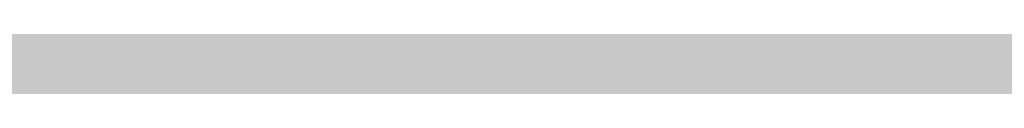
# Model space of a CAD drawing. Units: feet. Extents: x 3168 to 4724, y 827 to 1477.
# Tile 113 of 256: x 3284.48 to 3298.68, y 1098.34 to 1099. Entities that reach past the tile are written whole.
import ezdxf

# ---------------------------------------------------------------- set-up
doc = ezdxf.new("R2010")
doc.units = ezdxf.units.FT
doc.layers.add('A-ELEV', color=7, linetype='Continuous', lineweight=35)
doc.layers.add('A-ELEV-PATT', color=8, linetype='Continuous', lineweight=13)

msp = doc.modelspace()

# ---------------------------------------------------------------- hatches: boundary and pattern name
at = {"layer": 'A-ELEV-PATT'}
h = msp.add_hatch(color=256, dxfattribs=at)
h.dxf.hatch_style = 1
edge = h.paths.add_edge_path()
edge.add_ellipse((3552.906, 979.22), major_axis=(36.745, 0), ratio=0.484848, start_angle=0, end_angle=360)
edge = h.paths.add_edge_path()
edge.add_ellipse((3559.892, 929.252), major_axis=(36.745, 0), ratio=0.484848, start_angle=0, end_angle=360)
edge = h.paths.add_edge_path()
edge.add_line((3299.317, 1198.606), (3479.917, 1198.606))
edge.add_line((3479.917, 1198.606), (3479.917, 1209.869))
edge.add_spline(control_points=[(3479.917, 1209.869), (3464.301, 1209.869), (3448.686, 1209.869), (3410.949, 1209.869), (3388.828, 1209.869), (3355.647, 1209.869), (3344.586, 1209.869), (3327.996, 1209.869), (3322.466, 1209.869), (3314.17, 1209.869), (3311.405, 1209.869), (3307.257, 1209.869), (3305.875, 1209.869), (3303.801, 1209.869), (3303.11, 1209.869), (3302.073, 1209.869), (3301.727, 1209.869), (3301.209, 1209.869), (3301.036, 1209.869), (3300.777, 1209.869), (3300.69, 1209.869), (3300.561, 1209.869), (3300.517, 1209.869), (3300.453, 1209.869), (3300.431, 1209.869), (3300.399, 1209.869), (3300.388, 1209.869), (3300.366, 1209.869), (3300.346, 1209.869), (3300.346, 1209.869), (3300.346, 1209.869), (3300.343, 1209.869), (3300.341, 1209.869), (3300.338, 1209.869), (3300.337, 1209.869), (3300.334, 1209.869), (3300.332, 1209.869), (3300.326, 1209.869), (3300.321, 1209.869), (3300.311, 1209.869), (3300.306, 1209.869), (3300.291, 1209.869), (3300.28, 1209.869), (3300.232, 1209.869), (3300.195, 1209.869), (3299.951, 1209.871), (3299.745, 1209.874), (3299.437, 1209.883), (3299.334, 1209.887), (3299.181, 1209.893), (3299.13, 1209.895), (3298.652, 1209.917), (3298.229, 1209.946), (3297.602, 1210.002), (3297.393, 1210.023), (3297.083, 1210.058), (3296.979, 1210.07), (3296.293, 1210.155), (3295.718, 1210.243), (3294.869, 1210.399), (3294.588, 1210.454), (3294.169, 1210.543), (3294.03, 1210.574), (3291.707, 1211.101), (3289.654, 1211.813), (3285.776, 1213.564), (3283.951, 1214.603), (3280.512, 1216.98), (3278.897, 1218.318), (3276.38, 1220.829), (3275.416, 1221.918), (3274.039, 1223.708), (3273.581, 1224.35), (3273.143, 1225.016)], knot_values=[39.119033, 39.119033, 39.119033, 39.119033, 39.286353, 39.286353, 39.523379, 39.523379, 39.641892, 39.641892, 39.701148, 39.701148, 39.730777, 39.730777, 39.745591, 39.745591, 39.752998, 39.752998, 39.756701, 39.756701, 39.758553, 39.758553, 39.759479, 39.759479, 39.759942, 39.759942, 39.760173, 39.760173, 39.760289, 39.760289, 39.760405, 39.760405, 39.760463, 39.760463, 39.763389, 39.763389, 39.764851, 39.764851, 39.767304, 39.767304, 39.773825, 39.773825, 39.78057, 39.78057, 39.79477, 39.79477, 39.845194, 39.845194, 40.126715, 40.126715, 40.267476, 40.267476, 40.337856, 40.337856, 40.927023, 40.927023, 41.221606, 41.221606, 41.368898, 41.368898, 42.202622, 42.202622, 42.619485, 42.619485, 42.827916, 42.827916, 46.118323, 46.118323, 49.408731, 49.408731, 52.699139, 52.699139, 54.927489, 54.927489, 56.104228, 56.104228, 56.104228, 56.104228], weights=[1, 1, 1, 1, 1, 1, 1, 1, 1, 1, 1, 1, 1, 1, 1, 1, 1, 1, 1, 1, 1, 1, 1, 1, 1, 1, 1, 1, 1, 1, 1, 1, 1, 1, 1, 1, 1, 1, 1, 1, 1, 1, 1, 1, 1, 1, 1, 1, 1, 1, 1, 1, 1, 1, 1, 1, 1, 1, 1, 1, 1, 1, 1, 1, 1, 1, 1, 1, 1, 1, 1, 1, 1, 1], degree=3, periodic=0)
edge.add_line((3273.143, 1225.016), (3273.143, 1099.016))
edge.add_line((3273.143, 1099.016), (3299.317, 1099.016))
edge.add_line((3299.317, 1099.016), (3299.317, 1198.606))
edge = h.paths.add_edge_path()
edge.add_line((3304.758, 1324.158), (3479.917, 1324.158))
edge.add_line((3479.917, 1324.158), (3479.917, 1335.715))
edge.add_line((3479.917, 1335.715), (3269.162, 1335.715))
edge.add_spline(control_points=[(3269.162, 1335.715), (3264.024, 1335.715), (3258.364, 1328.958), (3259.264, 1323.9)], knot_values=[0, 0, 0, 0, 15.412191, 15.412191, 15.412191, 15.412191], degree=3, periodic=0)
edge.add_line((3259.264, 1323.9), (3265.517, 1288.769))
edge.add_line((3265.517, 1288.769), (3275.265, 1261.546))
edge.add_line((3275.265, 1261.546), (3304.758, 1261.546))
edge.add_line((3304.758, 1261.546), (3304.758, 1324.158))
h = msp.add_hatch(color=256, dxfattribs=at)
h.dxf.hatch_style = 1
h.paths.add_polyline_path([(3384.525, 1099.016), (3335.029, 1099.016), (3299.317, 1099.016), (3273.143, 1099.016), (3217.565, 1099.016), (3168.069, 827.116), (3335.029, 827.116)])

# ---------------------------------------------------------------- linework, layer by layer
at = {"layer": 'A-ELEV'}
msp.add_open_spline([(3808.52, 1099.016), (3808.52, 1141.413), (3808.52, 1183.81), (3808.52, 1226.635), (3808.52, 1227.064), (3808.52, 1227.492), (3811.492, 1248.995), (3814.464, 1270.498), (3817.465, 1292.218), (3817.495, 1292.435), (3817.525, 1292.652), (3817.573, 1310.107), (3817.62, 1327.562), (3817.668, 1345.016), (3817.668, 1345.458), (3817.668, 1345.9), (3817.668, 1346.456), (3817.668, 1346.571), (3817.668, 1346.753), (3817.668, 1346.82), (3817.668, 1346.935), (3817.668, 1346.982), (3817.668, 1347.039), (3817.668, 1347.047), (3817.668, 1347.074), (3817.668, 1347.059), (3817.668, 1347.062), (3817.668, 1347.063), (3817.668, 1347.066), (3817.668, 1347.068), (3817.668, 1347.075), (3817.668, 1347.079), (3817.668, 1347.093), (3817.668, 1347.102), (3817.668, 1347.129), (3817.668, 1347.147), (3817.667, 1347.2), (3817.667, 1347.236), (3817.666, 1347.343), (3817.665, 1347.415), (3817.661, 1347.628), (3817.657, 1347.77), (3817.64, 1348.192), (3817.624, 1348.472), (3817.559, 1349.3), (3817.496, 1349.841), (3817.255, 1351.424), (3817.026, 1352.429), (3816.307, 1354.889), (3815.744, 1356.269), (3814.464, 1358.819), (3813.746, 1359.991), (3812.196, 1362.172), (3811.362, 1363.182), (3809.589, 1365.069), (3808.649, 1365.946), (3806.654, 1367.58), (3805.6, 1368.336), (3803.353, 1369.722), (3802.161, 1370.352), (3799.601, 1371.454), (3798.233, 1371.925), (3795.28, 1372.635), (3793.693, 1372.872), (3791.869, 1372.926), (3791.741, 1372.929), (3791.353, 1372.934), (3791.093, 1372.933), (3790.304, 1372.915), (3789.77, 1372.884), (3789.209, 1372.83), (3789.191, 1372.828), (3789.135, 1372.823), (3789.098, 1372.819), (3789.048, 1372.814), (3789.036, 1372.813), (3789, 1372.809), (3788.976, 1372.806), (3788.949, 1372.803), (3788.947, 1372.803), (3788.943, 1372.803), (3788.941, 1372.802), (3788.939, 1372.802), (3788.938, 1372.802), (3788.935, 1372.802), (3788.868, 1372.794), (3788.757, 1372.782), (3788.702, 1372.776), (3788.536, 1372.758), (3788.425, 1372.746), (3788.093, 1372.709), (3787.872, 1372.685), (3787.208, 1372.612), (3786.765, 1372.563), (3785.437, 1372.417), (3784.551, 1372.32), (3781.895, 1372.027), (3780.125, 1371.833), (3774.813, 1371.248), (3771.271, 1370.859), (3760.647, 1369.69), (3753.564, 1368.911), (3732.316, 1366.573), (3718.15, 1365.015), (3694.007, 1362.359), (3684.029, 1361.262), (3674.051, 1360.164), (3664.601, 1360.164), (3655.151, 1360.164), (3626.801, 1360.164), (3607.901, 1360.164), (3551.202, 1360.164), (3513.402, 1360.164), (3467.725, 1360.164), (3459.848, 1360.164), (3436.215, 1360.164), (3420.46, 1360.164), (3373.194, 1360.164), (3341.684, 1360.164), (3302.848, 1360.164), (3295.523, 1360.164), (3286.038, 1360.164), (3283.879, 1360.164), (3277.403, 1360.164), (3273.085, 1360.164), (3267.733, 1360.164), (3266.699, 1360.164), (3263.597, 1360.164), (3261.528, 1360.164), (3259.237, 1360.164), (3259.014, 1360.164), (3258.344, 1360.164), (3257.897, 1360.164), (3257.431, 1360.164), (3257.411, 1360.164), (3257.371, 1360.164), (3257.375, 1360.164), (3257.375, 1360.164), (3257.374, 1360.164), (3257.372, 1360.164), (3257.371, 1360.164), (3257.367, 1360.164), (3257.364, 1360.164), (3257.356, 1360.164), (3257.351, 1360.164), (3257.335, 1360.164), (3257.324, 1360.164), (3257.293, 1360.164), (3257.272, 1360.164), (3257.208, 1360.163), (3257.166, 1360.163), (3257.04, 1360.161), (3256.956, 1360.16), (3256.706, 1360.153), (3256.539, 1360.147), (3256.044, 1360.122), (3255.717, 1360.097), (3254.752, 1360), (3254.128, 1359.907), (3252.18, 1359.525), (3250.942, 1359.144), (3248.67, 1358.243), (3247.636, 1357.724), (3245.733, 1356.603), (3244.863, 1356.002), (3243.253, 1354.743), (3242.512, 1354.085), (3240.751, 1352.345), (3239.801, 1351.23), (3238.088, 1348.872), (3237.325, 1347.63), (3235.983, 1344.972), (3235.402, 1343.555), (3234.591, 1340.815), (3234.311, 1339.544), (3233.976, 1336.803), (3233.922, 1335.331), (3234.149, 1332.591), (3234.35, 1331.367), (3234.72, 1329.999), (3234.752, 1329.883), (3234.854, 1329.535), (3234.926, 1329.302), (3235.025, 1329.003), (3235.047, 1328.937), (3235.078, 1328.847), (3235.086, 1328.823), (3235.111, 1328.751), (3235.128, 1328.703), (3235.148, 1328.646), (3235.151, 1328.638), (3235.156, 1328.624), (3235.158, 1328.618), (3235.16, 1328.612), (3235.166, 1328.597), (3235.18, 1328.556), (3235.19, 1328.528), (3235.221, 1328.443), (3235.241, 1328.386), (3235.302, 1328.216), (3235.343, 1328.102), (3235.465, 1327.762), (3235.546, 1327.535), (3235.79, 1326.853), (3235.953, 1326.399), (3236.44, 1325.037), (3236.766, 1324.128), (3237.741, 1321.403), (3238.392, 1319.587), (3240.344, 1314.137), (3241.645, 1310.504), (3245.548, 1299.604), (3248.15, 1292.337), (3255.956, 1270.537), (3261.16, 1256.004), (3267.388, 1238.612), (3268.411, 1235.753), (3269.51, 1232.684), (3269.586, 1232.474), (3269.707, 1232.136), (3269.752, 1232.008), (3269.827, 1231.799), (3269.856, 1231.718), (3269.906, 1231.578), (3269.927, 1231.52), (3269.972, 1231.393), (3269.997, 1231.325), (3270.027, 1231.243), (3270.032, 1231.228), (3270.04, 1231.204), (3270.039, 1231.207), (3270.039, 1231.207), (3270.039, 1231.206), (3270.04, 1231.206), (3270.04, 1231.205), (3270.04, 1231.204), (3270.04, 1231.204), (3270.041, 1231.201), (3270.042, 1231.2), (3270.043, 1231.195), (3270.045, 1231.192), (3270.048, 1231.183), (3270.05, 1231.177), (3270.056, 1231.159), (3270.061, 1231.147), (3270.074, 1231.111), (3270.083, 1231.087), (3270.109, 1231.014), (3270.127, 1230.966), (3270.18, 1230.822), (3270.216, 1230.727), (3270.325, 1230.442), (3270.4, 1230.253), (3270.629, 1229.691), (3270.789, 1229.324), (3271.286, 1228.238), (3271.643, 1227.54), (3272.776, 1225.515), (3273.614, 1224.261), (3275.416, 1221.918), (3276.38, 1220.829), (3278.897, 1218.318), (3280.512, 1216.98), (3283.951, 1214.603), (3285.776, 1213.564), (3289.654, 1211.813), (3291.707, 1211.101), (3294.03, 1210.574), (3294.169, 1210.543), (3294.588, 1210.454), (3294.869, 1210.399), (3295.718, 1210.243), (3296.293, 1210.155), (3296.979, 1210.07), (3297.083, 1210.058), (3297.393, 1210.023), (3297.602, 1210.002), (3298.229, 1209.946), (3298.652, 1209.917), (3299.13, 1209.895), (3299.181, 1209.893), (3299.334, 1209.887), (3299.437, 1209.883), (3299.745, 1209.874), (3299.951, 1209.871), (3300.195, 1209.869), (3300.232, 1209.869), (3300.28, 1209.869), (3300.291, 1209.869), (3300.306, 1209.869), (3300.311, 1209.869), (3300.321, 1209.869), (3300.326, 1209.869), (3300.332, 1209.869), (3300.334, 1209.869), (3300.337, 1209.869), (3300.338, 1209.869), (3300.341, 1209.869), (3300.343, 1209.869), (3300.346, 1209.869), (3300.346, 1209.869), (3300.346, 1209.869), (3300.366, 1209.869), (3300.388, 1209.869), (3300.399, 1209.869), (3300.431, 1209.869), (3300.453, 1209.869), (3300.517, 1209.869), (3300.561, 1209.869), (3300.69, 1209.869), (3300.777, 1209.869), (3301.036, 1209.869), (3301.209, 1209.869), (3301.727, 1209.869), (3302.073, 1209.869), (3303.11, 1209.869), (3303.801, 1209.869), (3305.875, 1209.869), (3307.257, 1209.869), (3311.405, 1209.869), (3314.17, 1209.869), (3322.466, 1209.869), (3327.996, 1209.869), (3344.586, 1209.869), (3355.647, 1209.869), (3388.828, 1209.869), (3410.949, 1209.869), (3477.312, 1209.869), (3521.554, 1209.869), (3566.836, 1209.869), (3567.877, 1209.869), (3570.999, 1209.869), (3573.08, 1209.869), (3575.781, 1209.869), (3576.401, 1209.869), (3577.296, 1209.869), (3577.571, 1209.869), (3578.397, 1209.869), (3578.948, 1209.869), (3579.756, 1209.869), (3580.015, 1209.869), (3580.343, 1209.869), (3580.327, 1209.869), (3580.327, 1209.869), (3580.327, 1209.869), (3580.328, 1209.869), (3580.328, 1209.869), (3580.329, 1209.869), (3580.33, 1209.869), (3580.331, 1209.869), (3580.333, 1209.869), (3580.336, 1209.869), (3580.339, 1209.869), (3580.346, 1209.869), (3580.351, 1209.869), (3580.366, 1209.869), (3580.375, 1209.869), (3580.405, 1209.868), (3580.424, 1209.868), (3580.483, 1209.868), (3580.522, 1209.868), (3580.64, 1209.867), (3580.719, 1209.865), (3580.956, 1209.861), (3581.115, 1209.856), (3581.594, 1209.837), (3581.916, 1209.818), (3582.89, 1209.742), (3583.548, 1209.666), (3585.532, 1209.361), (3586.867, 1209.054), (3589.472, 1208.252), (3590.74, 1207.758), (3591.995, 1207.159), (3592.058, 1207.129), (3592.244, 1207.038), (3592.368, 1206.977), (3592.735, 1206.79), (3592.977, 1206.663), (3593.245, 1206.516), (3593.275, 1206.5), (3593.365, 1206.45), (3593.425, 1206.416), (3593.604, 1206.315), (3593.723, 1206.247), (3593.857, 1206.168), (3593.874, 1206.158), (3593.926, 1206.128), (3593.96, 1206.108), (3594.062, 1206.047), (3594.13, 1206.006), (3594.208, 1205.958), (3594.22, 1205.951), (3594.253, 1205.931), (3594.276, 1205.917), (3594.343, 1205.876), (3594.388, 1205.848), (3594.434, 1205.819), (3594.435, 1205.818), (3594.44, 1205.815), (3594.443, 1205.813), (3594.447, 1205.811), (3594.448, 1205.81), (3594.449, 1205.81), (3594.449, 1205.809), (3594.45, 1205.809), (3594.45, 1205.808), (3594.451, 1205.808), (3594.467, 1205.798), (3594.493, 1205.782), (3594.506, 1205.774), (3594.545, 1205.749), (3594.571, 1205.733), (3594.648, 1205.684), (3594.7, 1205.652), (3594.855, 1205.555), (3594.959, 1205.49), (3595.269, 1205.295), (3595.476, 1205.166), (3596.097, 1204.776), (3596.511, 1204.517), (3597.753, 1203.739), (3598.581, 1203.22), (3601.064, 1201.664), (3602.72, 1200.626), (3607.687, 1197.513), (3610.998, 1195.438), (3620.932, 1189.212), (3627.555, 1185.061), (3647.423, 1172.61), (3660.668, 1164.309), (3700.403, 1139.405), (3726.894, 1122.803), (3757.206, 1103.806), (3761.027, 1101.411), (3764.848, 1099.016), (3745.328, 1099.016), (3725.808, 1099.016), (3706.288, 1099.016), (3706.288, 1108.453), (3706.288, 1117.89), (3706.288, 1127.327), (3710.751, 1127.327), (3715.213, 1127.327), (3719.676, 1127.327)], degree=3, knots=[0, 0, 0, 0, 0.982037, 0.982037, 0.991957, 0.991957, 0.991957, 1.966522, 1.966522, 1.976367, 1.976367, 1.976367, 2.976367, 2.976367, 2.976367, 3.00169, 3.00169, 3.008272, 3.008272, 3.012129, 3.012129, 3.014851, 3.014851, 3.015353, 3.015353, 3.016359, 3.016359, 3.017365, 3.017365, 3.019376, 3.019376, 3.023398, 3.023398, 3.031442, 3.031442, 3.047531, 3.047531, 3.079708, 3.079708, 3.144063, 3.144063, 3.272772, 3.272772, 3.53019, 3.53019, 4.045026, 4.045026, 5.074698, 5.074698, 6.700878, 6.700878, 8.327058, 8.327058, 9.953238, 9.953238, 11.579418, 11.579418, 13.205598, 13.205598, 14.831778, 14.831778, 16.457958, 16.457958, 18.084138, 18.084138, 18.206872, 18.206872, 18.45234, 18.45234, 18.943275, 18.943275, 18.960093, 18.960093, 18.993729, 18.993729, 19.00461, 19.00461, 19.026374, 19.026374, 19.028737, 19.028737, 19.03018, 19.03018, 19.030897, 19.030897, 19.032332, 19.032332, 19.033766, 19.033766, 19.036636, 19.036636, 19.042374, 19.042374, 19.053851, 19.053851, 19.076805, 19.076805, 19.122714, 19.122714, 19.21453, 19.21453, 19.398163, 19.398163, 19.765429, 19.765429, 20.024128, 20.024128, 20.024128, 20.092031, 20.092031, 20.227836, 20.227836, 20.499446, 20.499446, 20.556051, 20.556051, 20.66926, 20.66926, 20.895678, 20.895678, 20.948316, 20.948316, 20.963829, 20.963829, 20.994855, 20.994855, 21.002285, 21.002285, 21.017146, 21.017146, 21.01875, 21.01875, 21.021959, 21.021959, 21.022102, 21.022102, 21.022249, 21.022249, 21.022708, 21.022708, 21.023627, 21.023627, 21.025464, 21.025464, 21.029138, 21.029138, 21.036486, 21.036486, 21.051183, 21.051183, 21.080575, 21.080575, 21.139361, 21.139361, 21.256932, 21.256932, 21.492073, 21.492073, 21.962356, 21.962356, 23.01002, 23.01002, 24.057684, 24.057684, 25.105348, 25.105348, 26.153011, 26.153011, 27.776787, 27.776787, 29.400562, 29.400562, 31.024337, 31.024337, 32.278801, 32.278801, 33.533265, 33.533265, 34.467568, 34.467568, 34.553971, 34.553971, 34.726776, 34.726776, 34.775309, 34.775309, 34.793079, 34.793079, 34.82862, 34.82862, 34.834979, 34.834979, 34.839039, 34.839039, 34.839411, 34.839411, 34.840285, 34.840285, 34.842034, 34.842034, 34.845531, 34.845531, 34.852525, 34.852525, 34.866512, 34.866512, 34.894488, 34.894488, 34.950439, 34.950439, 35.062342, 35.062342, 35.286147, 35.286147, 35.733758, 35.733758, 35.821815, 35.821815, 35.828283, 35.828283, 35.832225, 35.832225, 35.834724, 35.834724, 35.836521, 35.836521, 35.838617, 35.838617, 35.839073, 35.839073, 35.839345, 35.839345, 35.839617, 35.839617, 35.840161, 35.840161, 35.841249, 35.841249, 35.843425, 35.843425, 35.847778, 35.847778, 35.856482, 35.856482, 35.873891, 35.873891, 35.908709, 35.908709, 35.978345, 35.978345, 36.117617, 36.117617, 36.396161, 36.396161, 36.953248, 36.953248, 38.067423, 38.067423, 40.295772, 40.295772, 42.524122, 42.524122, 45.81453, 45.81453, 49.104937, 49.104937, 52.395345, 52.395345, 52.603776, 52.603776, 53.020639, 53.020639, 53.854363, 53.854363, 54.001655, 54.001655, 54.296238, 54.296238, 54.885405, 54.885405, 54.955785, 54.955785, 55.096546, 55.096546, 55.378067, 55.378067, 55.42849, 55.42849, 55.442691, 55.442691, 55.449436, 55.449436, 55.455957, 55.455957, 55.458409, 55.458409, 55.459872, 55.459872, 55.462798, 55.462798, 55.462856, 55.462856, 55.462972, 55.462972, 55.463088, 55.463088, 55.463319, 55.463319, 55.463782, 55.463782, 55.464708, 55.464708, 55.46656, 55.46656, 55.470263, 55.470263, 55.47767, 55.47767, 55.492484, 55.492484, 55.522112, 55.522112, 55.581369, 55.581369, 55.699882, 55.699882, 55.936907, 55.936907, 56.410959, 56.410959, 56.42211, 56.42211, 56.444413, 56.444413, 56.451051, 56.451051, 56.454001, 56.454001, 56.459901, 56.459901, 56.462666, 56.462666, 56.463418, 56.463418, 56.464171, 56.464171, 56.465675, 56.465675, 56.468684, 56.468684, 56.474702, 56.474702, 56.486738, 56.486738, 56.51081, 56.51081, 56.558955, 56.558955, 56.655243, 56.655243, 56.847821, 56.847821, 57.232975, 57.232975, 58.003284, 58.003284, 59.543901, 59.543901, 62.625137, 62.625137, 68.787607, 68.787607, 74.950078, 74.950078, 75.27336, 75.27336, 75.919923, 75.919923, 77.213051, 77.213051, 77.377769, 77.377769, 77.707206, 77.707206, 78.366079, 78.366079, 78.462532, 78.462532, 78.655436, 78.655436, 79.041245, 79.041245, 79.105735, 79.105735, 79.234714, 79.234714, 79.492672, 79.492672, 79.502197, 79.502197, 79.521249, 79.521249, 79.523534, 79.523534, 79.528103, 79.528103, 79.528682, 79.528682, 79.528885, 79.528885, 79.529089, 79.529089, 79.529495, 79.529495, 79.530308, 79.530308, 79.531935, 79.531935, 79.535187, 79.535187, 79.541693, 79.541693, 79.554704, 79.554704, 79.580725, 79.580725, 79.632769, 79.632769, 79.736856, 79.736856, 79.94503, 79.94503, 80.361377, 80.361377, 80.421435, 80.421435, 80.421435, 81.421435, 81.421435, 81.421435, 82.421435, 82.421435, 82.421435, 83.421435, 83.421435, 83.421435, 83.421435], dxfattribs=at)

doc.saveas('drawing.dxf')
